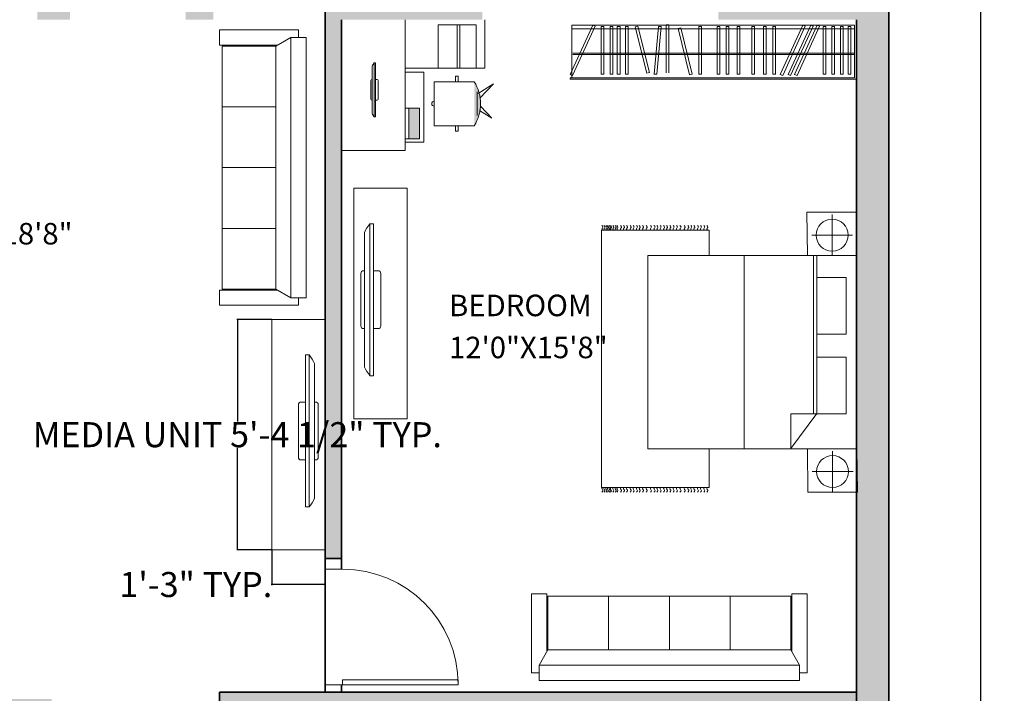
# Model space of a CAD drawing. Units: inches. Extents: x 1319 to 2030, y 219 to 1069.
# Tile 27 of 28: x 1727 to 2002, y 663 to 852. Entities that reach past the tile are written whole.
import ezdxf

# ---------------------------------------------------------------- set-up
doc = ezdxf.new("R2010")
doc.units = ezdxf.units.IN
doc.header["$MEASUREMENT"] = 0
doc.layers.get('0').update_dxf_attribs({"color": 12})
for name, color, linetype, lineweight in [('A-ANNO-DIMS', 2, 'Continuous', 18), ('A-AREA-IDEN', 250, 'Continuous', 18), ('A-WALL-PATT', 252, 'Continuous', 13), ('C-PROP', 7, 'Continuous', 35), ('closet', 252, 'Continuous', 18), ('doors', 252, 'Continuous', 18), ('furniture', 250, 'Continuous', 18), ('walls', 250, 'Continuous', 35)]:
    doc.layers.add(name, color=color, linetype=linetype, lineweight=lineweight)
doc.styles.get("Standard").update_dxf_attribs({"font": 'arial.ttf'})
doc.dimstyles.get("Standard").update_dxf_attribs({"dimtxt": 7, "dimasz": 0.18, "dimexe": 0.18, "dimexo": 0.0625, "dimgap": 0.09, "dimtad": 0, "dimtih": 1, "dimtoh": 1, "dimzin": 0, "dimdsep": 46, "dimlunit": 3, "dimtxsty": 'Standard', "dimcen": 0.09, "dimadec": 0, "dimazin": 0, "dimtfac": 1, "dimtofl": 0, "dimtmove": 0, "dimatfit": 3, "dimfxl": 1, "dimtolj": 1, "dimtzin": 0, "dimarcsym": 0})

# ---------------------------------------------------------------- blocks, each defined once
blk = doc.blocks.new('*U2')
for p, q in [((0, 0), (0, -6)), ((40, 0), (40, -6))]:
    blk.add_line(p, q)
blk.add_lwpolyline([(0, 0), (0, 40), (1.75, 40), (1.75, 0)], close=True)
blk.add_arc((0, 0), 40, 0, 90)
blk = doc.blocks.new('CARPET')
at = {"layer": 'furniture'}
for p, q in [((-51.53, -98.11), (-51.53, -55.12)), ((-51.53, -55.12), (-41.27, -55.12)), ((36, -55.12), (51.55, -55.12)), ((51.55, -55.12), (51.55, -98.11)), ((51.55, -98.11), (-51.53, -98.11))]:
    blk.add_line(p, q, dxfattribs=at)
for points, knots in [([(-53.37, -55.99), (-53.22, -55.8), (-52.9, -55.41), (-52.34, -55.8), (-51.89, -56.08), (-51.65, -55.91), (-51.53, -55.83)], [0, 0, 0, 0, 0.653278, 1.290138, 1.740457, 2.114451, 2.114451, 2.114451, 2.114451]), ([(-53.37, -57.26), (-53.22, -57.07), (-52.9, -56.67), (-52.34, -57.07), (-51.89, -57.35), (-51.65, -57.17), (-51.53, -57.1)], [0, 0, 0, 0, 0.653278, 1.290138, 1.740457, 2.114451, 2.114451, 2.114451, 2.114451]), ([(-53.37, -58.59), (-53.22, -58.4), (-52.9, -58.01), (-52.34, -58.4), (-51.89, -58.68), (-51.65, -58.5), (-51.53, -58.43)], [0, 0, 0, 0, 0.653278, 1.290138, 1.740457, 2.114451, 2.114451, 2.114451, 2.114451]), ([(53.37, -55.99), (53.22, -55.8), (52.9, -55.41), (52.34, -55.8), (51.89, -56.08), (51.65, -55.91), (51.53, -55.83)], [0, 0, 0, 0, 0.653278, 1.290138, 1.740457, 2.114451, 2.114451, 2.114451, 2.114451]), ([(53.37, -57.26), (53.22, -57.07), (52.9, -56.67), (52.34, -57.07), (51.89, -57.35), (51.65, -57.17), (51.53, -57.1)], [0, 0, 0, 0, 0.653278, 1.290138, 1.740457, 2.114451, 2.114451, 2.114451, 2.114451]), ([(53.37, -58.59), (53.22, -58.4), (52.9, -58.01), (52.34, -58.4), (51.89, -58.68), (51.65, -58.5), (51.53, -58.43)], [0, 0, 0, 0, 0.653278, 1.290138, 1.740457, 2.114451, 2.114451, 2.114451, 2.114451]), ([(-53.37, -59.78), (-53.22, -59.58), (-52.9, -59.19), (-52.34, -59.58), (-51.89, -59.86), (-51.65, -59.69), (-51.53, -59.61)], [0, 0, 0, 0, 0.653278, 1.290138, 1.740457, 2.114451, 2.114451, 2.114451, 2.114451]), ([(-53.37, -61.22), (-53.22, -61.02), (-52.9, -60.63), (-52.34, -61.02), (-51.89, -61.3), (-51.65, -61.13), (-51.53, -61.05)], [0, 0, 0, 0, 0.653278, 1.290138, 1.740457, 2.114451, 2.114451, 2.114451, 2.114451]), ([(-53.37, -62.44), (-53.22, -62.25), (-52.9, -61.86), (-52.34, -62.25), (-51.89, -62.53), (-51.65, -62.36), (-51.53, -62.28)], [0, 0, 0, 0, 0.653278, 1.290138, 1.740457, 2.114451, 2.114451, 2.114451, 2.114451]), ([(53.37, -59.78), (53.22, -59.58), (52.9, -59.19), (52.34, -59.58), (51.89, -59.86), (51.65, -59.69), (51.53, -59.61)], [0, 0, 0, 0, 0.653278, 1.290138, 1.740457, 2.114451, 2.114451, 2.114451, 2.114451]), ([(53.37, -61.22), (53.22, -61.02), (52.9, -60.63), (52.34, -61.02), (51.89, -61.3), (51.65, -61.13), (51.53, -61.05)], [0, 0, 0, 0, 0.653278, 1.290138, 1.740457, 2.114451, 2.114451, 2.114451, 2.114451]), ([(53.37, -62.44), (53.22, -62.25), (52.9, -61.86), (52.34, -62.25), (51.89, -62.53), (51.65, -62.36), (51.53, -62.28)], [0, 0, 0, 0, 0.653278, 1.290138, 1.740457, 2.114451, 2.114451, 2.114451, 2.114451]), ([(-53.37, -63.63), (-53.22, -63.43), (-52.9, -63.04), (-52.34, -63.43), (-51.89, -63.72), (-51.65, -63.54), (-51.53, -63.46)], [0, 0, 0, 0, 0.653278, 1.290138, 1.740457, 2.114451, 2.114451, 2.114451, 2.114451]), ([(-53.37, -65.07), (-53.22, -64.87), (-52.9, -64.48), (-52.34, -64.87), (-51.89, -65.15), (-51.65, -64.98), (-51.53, -64.9)], [0, 0, 0, 0, 0.653278, 1.290138, 1.740457, 2.114451, 2.114451, 2.114451, 2.114451]), ([(-53.37, -66.76), (-53.22, -66.56), (-52.9, -66.17), (-52.34, -66.56), (-51.89, -66.84), (-51.65, -66.67), (-51.53, -66.59)], [0, 0, 0, 0, 0.653278, 1.290138, 1.740457, 2.114451, 2.114451, 2.114451, 2.114451]), ([(53.37, -63.63), (53.22, -63.43), (52.9, -63.04), (52.34, -63.43), (51.89, -63.72), (51.65, -63.54), (51.53, -63.46)], [0, 0, 0, 0, 0.653278, 1.290138, 1.740457, 2.114451, 2.114451, 2.114451, 2.114451]), ([(53.37, -65.07), (53.22, -64.87), (52.9, -64.48), (52.34, -64.87), (51.89, -65.15), (51.65, -64.98), (51.53, -64.9)], [0, 0, 0, 0, 0.653278, 1.290138, 1.740457, 2.114451, 2.114451, 2.114451, 2.114451]), ([(53.37, -66.76), (53.22, -66.56), (52.9, -66.17), (52.34, -66.56), (51.89, -66.84), (51.65, -66.67), (51.53, -66.59)], [0, 0, 0, 0, 0.653278, 1.290138, 1.740457, 2.114451, 2.114451, 2.114451, 2.114451]), ([(-53.37, -68.2), (-53.22, -68), (-52.9, -67.61), (-52.34, -68), (-51.89, -68.28), (-51.65, -68.11), (-51.53, -68.03)], [0, 0, 0, 0, 0.653278, 1.290138, 1.740457, 2.114451, 2.114451, 2.114451, 2.114451]), ([(-53.37, -69.53), (-53.22, -69.33), (-52.9, -68.94), (-52.34, -69.33), (-51.89, -69.61), (-51.65, -69.44), (-51.53, -69.36)], [0, 0, 0, 0, 0.653278, 1.290138, 1.740457, 2.114451, 2.114451, 2.114451, 2.114451]), ([(-53.37, -70.79), (-53.22, -70.6), (-52.9, -70.21), (-52.34, -70.6), (-51.89, -70.88), (-51.65, -70.7), (-51.53, -70.63)], [0, 0, 0, 0, 0.653278, 1.290138, 1.740457, 2.114451, 2.114451, 2.114451, 2.114451]), ([(53.37, -68.2), (53.22, -68), (52.9, -67.61), (52.34, -68), (51.89, -68.28), (51.65, -68.11), (51.53, -68.03)], [0, 0, 0, 0, 0.653278, 1.290138, 1.740457, 2.114451, 2.114451, 2.114451, 2.114451]), ([(53.37, -69.53), (53.22, -69.33), (52.9, -68.94), (52.34, -69.33), (51.89, -69.61), (51.65, -69.44), (51.53, -69.36)], [0, 0, 0, 0, 0.653278, 1.290138, 1.740457, 2.114451, 2.114451, 2.114451, 2.114451]), ([(53.37, -70.79), (53.22, -70.6), (52.9, -70.21), (52.34, -70.6), (51.89, -70.88), (51.65, -70.7), (51.53, -70.63)], [0, 0, 0, 0, 0.653278, 1.290138, 1.740457, 2.114451, 2.114451, 2.114451, 2.114451]), ([(-53.37, -72.12), (-53.22, -71.93), (-52.9, -71.54), (-52.34, -71.93), (-51.89, -72.21), (-51.65, -72.04), (-51.53, -71.96)], [0, 0, 0, 0, 0.653278, 1.290138, 1.740457, 2.114451, 2.114451, 2.114451, 2.114451]), ([(-53.37, -73.31), (-53.22, -73.11), (-52.9, -72.72), (-52.34, -73.11), (-51.89, -73.4), (-51.65, -73.22), (-51.53, -73.14)], [0, 0, 0, 0, 0.653278, 1.290138, 1.740457, 2.114451, 2.114451, 2.114451, 2.114451]), ([(-53.37, -74.75), (-53.22, -74.55), (-52.9, -74.16), (-52.34, -74.55), (-51.89, -74.83), (-51.65, -74.66), (-51.53, -74.58)], [0, 0, 0, 0, 0.653278, 1.290138, 1.740457, 2.114451, 2.114451, 2.114451, 2.114451]), ([(53.37, -72.12), (53.22, -71.93), (52.9, -71.54), (52.34, -71.93), (51.89, -72.21), (51.65, -72.04), (51.53, -71.96)], [0, 0, 0, 0, 0.653278, 1.290138, 1.740457, 2.114451, 2.114451, 2.114451, 2.114451]), ([(53.37, -73.31), (53.22, -73.11), (52.9, -72.72), (52.34, -73.11), (51.89, -73.4), (51.65, -73.22), (51.53, -73.14)], [0, 0, 0, 0, 0.653278, 1.290138, 1.740457, 2.114451, 2.114451, 2.114451, 2.114451]), ([(53.37, -74.75), (53.22, -74.55), (52.9, -74.16), (52.34, -74.55), (51.89, -74.83), (51.65, -74.66), (51.53, -74.58)], [0, 0, 0, 0, 0.653278, 1.290138, 1.740457, 2.114451, 2.114451, 2.114451, 2.114451]), ([(-53.37, -75.98), (-53.22, -75.78), (-52.9, -75.39), (-52.34, -75.78), (-51.89, -76.06), (-51.65, -75.89), (-51.53, -75.81)], [0, 0, 0, 0, 0.653278, 1.290138, 1.740457, 2.114451, 2.114451, 2.114451, 2.114451]), ([(-53.37, -77.16), (-53.22, -76.96), (-52.9, -76.57), (-52.34, -76.96), (-51.89, -77.25), (-51.65, -77.07), (-51.53, -76.99)], [0, 0, 0, 0, 0.653278, 1.290138, 1.740457, 2.114451, 2.114451, 2.114451, 2.114451]), ([(-53.37, -78.6), (-53.22, -78.4), (-52.9, -78.01), (-52.34, -78.4), (-51.89, -78.68), (-51.65, -78.51), (-51.53, -78.43)], [0, 0, 0, 0, 0.653278, 1.290138, 1.740457, 2.114451, 2.114451, 2.114451, 2.114451]), ([(53.37, -75.98), (53.22, -75.78), (52.9, -75.39), (52.34, -75.78), (51.89, -76.06), (51.65, -75.89), (51.53, -75.81)], [0, 0, 0, 0, 0.653278, 1.290138, 1.740457, 2.114451, 2.114451, 2.114451, 2.114451]), ([(53.37, -77.16), (53.22, -76.96), (52.9, -76.57), (52.34, -76.96), (51.89, -77.25), (51.65, -77.07), (51.53, -76.99)], [0, 0, 0, 0, 0.653278, 1.290138, 1.740457, 2.114451, 2.114451, 2.114451, 2.114451]), ([(53.37, -78.6), (53.22, -78.4), (52.9, -78.01), (52.34, -78.4), (51.89, -78.68), (51.65, -78.51), (51.53, -78.43)], [0, 0, 0, 0, 0.653278, 1.290138, 1.740457, 2.114451, 2.114451, 2.114451, 2.114451]), ([(-53.37, -80.29), (-53.22, -80.09), (-52.9, -79.7), (-52.34, -80.09), (-51.89, -80.37), (-51.65, -80.2), (-51.53, -80.12)], [0, 0, 0, 0, 0.653278, 1.290138, 1.740457, 2.114451, 2.114451, 2.114451, 2.114451]), ([(-53.37, -81.73), (-53.22, -81.53), (-52.9, -81.14), (-52.34, -81.53), (-51.89, -81.81), (-51.65, -81.64), (-51.53, -81.56)], [0, 0, 0, 0, 0.653278, 1.290138, 1.740457, 2.114451, 2.114451, 2.114451, 2.114451]), ([(-53.37, -83.06), (-53.22, -82.86), (-52.9, -82.47), (-52.34, -82.86), (-51.89, -83.14), (-51.65, -82.97), (-51.53, -82.89)], [0, 0, 0, 0, 0.653278, 1.290138, 1.740457, 2.114451, 2.114451, 2.114451, 2.114451]), ([(53.37, -80.29), (53.22, -80.09), (52.9, -79.7), (52.34, -80.09), (51.89, -80.37), (51.65, -80.2), (51.53, -80.12)], [0, 0, 0, 0, 0.653278, 1.290138, 1.740457, 2.114451, 2.114451, 2.114451, 2.114451]), ([(53.37, -81.73), (53.22, -81.53), (52.9, -81.14), (52.34, -81.53), (51.89, -81.81), (51.65, -81.64), (51.53, -81.56)], [0, 0, 0, 0, 0.653278, 1.290138, 1.740457, 2.114451, 2.114451, 2.114451, 2.114451]), ([(53.37, -83.06), (53.22, -82.86), (52.9, -82.47), (52.34, -82.86), (51.89, -83.14), (51.65, -82.97), (51.53, -82.89)], [0, 0, 0, 0, 0.653278, 1.290138, 1.740457, 2.114451, 2.114451, 2.114451, 2.114451]), ([(-53.37, -84.18), (-53.22, -83.99), (-52.9, -83.6), (-52.34, -83.99), (-51.89, -84.27), (-51.65, -84.09), (-51.53, -84.02)], [0, 0, 0, 0, 0.653278, 1.290138, 1.740457, 2.114451, 2.114451, 2.114451, 2.114451]), ([(-53.37, -85.51), (-53.22, -85.32), (-52.9, -84.93), (-52.34, -85.32), (-51.89, -85.6), (-51.65, -85.42), (-51.53, -85.35)], [0, 0, 0, 0, 0.653278, 1.290138, 1.740457, 2.114451, 2.114451, 2.114451, 2.114451]), ([(-53.37, -86.7), (-53.22, -86.5), (-52.9, -86.11), (-52.34, -86.5), (-51.89, -86.78), (-51.65, -86.61), (-51.53, -86.53)], [0, 0, 0, 0, 0.653278, 1.290138, 1.740457, 2.114451, 2.114451, 2.114451, 2.114451]), ([(53.37, -84.18), (53.22, -83.99), (52.9, -83.6), (52.34, -83.99), (51.89, -84.27), (51.65, -84.09), (51.53, -84.02)], [0, 0, 0, 0, 0.653278, 1.290138, 1.740457, 2.114451, 2.114451, 2.114451, 2.114451]), ([(53.37, -85.51), (53.22, -85.32), (52.9, -84.93), (52.34, -85.32), (51.89, -85.6), (51.65, -85.42), (51.53, -85.35)], [0, 0, 0, 0, 0.653278, 1.290138, 1.740457, 2.114451, 2.114451, 2.114451, 2.114451]), ([(53.37, -86.7), (53.22, -86.5), (52.9, -86.11), (52.34, -86.5), (51.89, -86.78), (51.65, -86.61), (51.53, -86.53)], [0, 0, 0, 0, 0.653278, 1.290138, 1.740457, 2.114451, 2.114451, 2.114451, 2.114451]), ([(-53.37, -88.14), (-53.22, -87.94), (-52.9, -87.55), (-52.34, -87.94), (-51.89, -88.22), (-51.65, -88.05), (-51.53, -87.97)], [0, 0, 0, 0, 0.653278, 1.290138, 1.740457, 2.114451, 2.114451, 2.114451, 2.114451]), ([(-53.37, -89.36), (-53.22, -89.17), (-52.9, -88.78), (-52.34, -89.17), (-51.89, -89.45), (-51.65, -89.28), (-51.53, -89.2)], [0, 0, 0, 0, 0.653278, 1.290138, 1.740457, 2.114451, 2.114451, 2.114451, 2.114451]), ([(-53.37, -90.55), (-53.22, -90.35), (-52.9, -89.96), (-52.34, -90.35), (-51.89, -90.64), (-51.65, -90.46), (-51.53, -90.38)], [0, 0, 0, 0, 0.653278, 1.290138, 1.740457, 2.114451, 2.114451, 2.114451, 2.114451]), ([(53.37, -88.14), (53.22, -87.94), (52.9, -87.55), (52.34, -87.94), (51.89, -88.22), (51.65, -88.05), (51.53, -87.97)], [0, 0, 0, 0, 0.653278, 1.290138, 1.740457, 2.114451, 2.114451, 2.114451, 2.114451]), ([(53.37, -89.36), (53.22, -89.17), (52.9, -88.78), (52.34, -89.17), (51.89, -89.45), (51.65, -89.28), (51.53, -89.2)], [0, 0, 0, 0, 0.653278, 1.290138, 1.740457, 2.114451, 2.114451, 2.114451, 2.114451]), ([(53.37, -90.55), (53.22, -90.35), (52.9, -89.96), (52.34, -90.35), (51.9, -90.63), (51.66, -90.47), (51.55, -90.4)], [0, 0, 0, 0, 0.653278, 1.290138, 1.740457, 2.0926, 2.0926, 2.0926, 2.0926]), ([(-53.37, -91.99), (-53.22, -91.79), (-52.9, -91.4), (-52.34, -91.79), (-51.89, -92.07), (-51.65, -91.9), (-51.53, -91.82)], [0, 0, 0, 0, 0.653278, 1.290138, 1.740457, 2.114451, 2.114451, 2.114451, 2.114451]), ([(-53.37, -92.69), (-53.22, -92.48), (-52.9, -92.08), (-52.35, -92.49), (-51.89, -92.77), (-51.65, -92.6), (-51.53, -92.52)], [0, 0, 0, 0, 0.663904, 1.307406, 1.757725, 2.131719, 2.131719, 2.131719, 2.131719]), ([(-53.37, -93.61), (-53.22, -93.42), (-52.9, -93.03), (-52.34, -93.42), (-51.89, -93.7), (-51.65, -93.52), (-51.53, -93.45)], [0, 0, 0, 0, 0.653278, 1.290138, 1.740457, 2.114451, 2.114451, 2.114451, 2.114451]), ([(-53.37, -94.55), (-53.22, -94.35), (-52.9, -93.96), (-52.34, -94.35), (-51.89, -94.63), (-51.65, -94.46), (-51.53, -94.38)], [0, 0, 0, 0, 0.653278, 1.290138, 1.740457, 2.114451, 2.114451, 2.114451, 2.114451]), ([(53.37, -91.99), (53.22, -91.79), (52.9, -91.4), (52.34, -91.79), (51.9, -92.07), (51.66, -91.91), (51.55, -91.83)], [0, 0, 0, 0, 0.653278, 1.290138, 1.740457, 2.0926, 2.0926, 2.0926, 2.0926]), ([(53.37, -92.69), (53.22, -92.49), (52.9, -92.09), (52.34, -92.49), (51.9, -92.77), (51.66, -92.61), (51.55, -92.53)], [0, 0, 0, 0, 0.656792, 1.295826, 1.746145, 2.098292, 2.098292, 2.098292, 2.098292]), ([(53.37, -93.66), (53.22, -93.46), (52.9, -93.07), (52.34, -93.46), (51.9, -93.74), (51.66, -93.58), (51.55, -93.5)], [0, 0, 0, 0, 0.653278, 1.290138, 1.740457, 2.0926, 2.0926, 2.0926, 2.0926]), ([(53.37, -94.59), (53.22, -94.4), (52.9, -94.01), (52.34, -94.4), (51.9, -94.68), (51.66, -94.51), (51.55, -94.44)], [0, 0, 0, 0, 0.653278, 1.290138, 1.740457, 2.0926, 2.0926, 2.0926, 2.0926]), ([(-53.37, -95.05), (-53.22, -94.85), (-52.9, -94.46), (-52.34, -94.85), (-51.89, -95.14), (-51.65, -94.96), (-51.53, -94.88)], [0, 0, 0, 0, 0.653278, 1.290138, 1.740457, 2.114451, 2.114451, 2.114451, 2.114451]), ([(-53.37, -95.73), (-53.22, -95.54), (-52.9, -95.15), (-52.34, -95.54), (-51.89, -95.82), (-51.65, -95.65), (-51.53, -95.57)], [0, 0, 0, 0, 0.653278, 1.290138, 1.740457, 2.114451, 2.114451, 2.114451, 2.114451]), ([(-53.37, -96.38), (-53.22, -96.18), (-52.9, -95.79), (-52.34, -96.18), (-51.89, -96.47), (-51.65, -96.29), (-51.53, -96.21)], [0, 0, 0, 0, 0.653278, 1.290138, 1.740457, 2.114451, 2.114451, 2.114451, 2.114451]), ([(-53.37, -97.17), (-53.22, -96.98), (-52.9, -96.59), (-52.34, -96.98), (-51.89, -97.26), (-51.65, -97.08), (-51.53, -97.01)], [0, 0, 0, 0, 0.653278, 1.290138, 1.740457, 2.114451, 2.114451, 2.114451, 2.114451]), ([(-53.37, -97.99), (-53.22, -97.79), (-52.9, -97.4), (-52.34, -97.79), (-51.89, -98.08), (-51.65, -97.9), (-51.53, -97.82)], [0, 0, 0, 0, 0.653278, 1.290138, 1.740457, 2.114451, 2.114451, 2.114451, 2.114451]), ([(53.37, -95.78), (53.22, -95.58), (52.9, -95.19), (52.34, -95.58), (51.89, -95.86), (51.65, -95.69), (51.53, -95.61)], [0, 0, 0, 0, 0.653278, 1.290138, 1.740457, 2.114451, 2.114451, 2.114451, 2.114451]), ([(53.37, -96.43), (53.22, -96.23), (52.9, -95.84), (52.34, -96.23), (51.89, -96.51), (51.65, -96.34), (51.53, -96.26)], [0, 0, 0, 0, 0.653278, 1.290138, 1.740457, 2.114451, 2.114451, 2.114451, 2.114451]), ([(53.37, -97.22), (53.22, -97.02), (52.9, -96.63), (52.34, -97.02), (51.89, -97.3), (51.65, -97.13), (51.53, -97.05)], [0, 0, 0, 0, 0.653278, 1.290138, 1.740457, 2.114451, 2.114451, 2.114451, 2.114451]), ([(53.37, -97.99), (53.22, -97.79), (52.9, -97.4), (52.34, -97.79), (51.89, -98.08), (51.65, -97.9), (51.53, -97.82)], [0, 0, 0, 0, 0.653278, 1.290138, 1.740457, 2.114451, 2.114451, 2.114451, 2.114451]), ([(53.37, -95.1), (53.22, -94.9), (52.9, -94.51), (52.34, -94.9), (51.9, -95.18), (51.66, -95.02), (51.55, -94.94)], [0, 0, 0, 0, 0.653278, 1.290138, 1.740457, 2.0926, 2.0926, 2.0926, 2.0926])]:
    blk.add_open_spline(points, degree=3, knots=knots, dxfattribs=at)
blk = doc.blocks.new('A$C58D270C6')
at = {"layer": 'furniture'}
for p, q in [((9.09, 124.13), (9.09, 108.87)), ((1.46, 116.5), (16.73, 116.5)), ((14.97, 94.84), (24.62, 107.92)), ((24.62, 94.93), (24.62, 107.92)), ((42.08, 108), (42.08, 36)), ((14.97, 94.93), (24.62, 94.93)), ((14.97, 94.84), (14.97, 36)), ((16.22, 94.93), (16.22, 36)), ((9.25, 36), (9.25, 20.74)), ((1.62, 28.37), (16.88, 28.37))]:
    blk.add_line(p, q, dxfattribs=at)
for points in [[(18.5, 108), (18.34, 124.13), (-0.16, 124.13), (0, 108)], [(0, 108), (77.91, 108), (77.91, 36), (0, 36)], [(4.09, 94.93), (14.97, 94.93), (14.97, 73.83), (4.09, 73.83)], [(4.09, 65.23), (14.97, 65.23), (14.97, 44.13), (4.09, 44.13)], [(18.65, 19.87), (18.5, 36), (0, 36), (0.16, 19.87)]]:
    blk.add_lwpolyline(points, close=True, dxfattribs=at)
for centre in [(9.09, 116.5), (9.25, 28.37)]:
    blk.add_circle(centre, 5.95, dxfattribs=at)
at = {"layer": 'furniture', "xscale": 0.9312884925094044, "yscale": 0.9312884925094044, "zscale": 0.9312884925094044, "rotation": 90}
blk.add_blockref('CARPET', (3.79, 74.47), dxfattribs=at)
blk = doc.blocks.new('FABRIC SOFA 4S')
at = {"layer": 'furniture'}
for p, q in [((0, -51), (0, 51)), ((6, 51), (0, 51)), ((3, 54), (34, 54)), ((3, 51), (3, 54)), ((6, -51), (6, 51)), ((12, 47.63), (6, 51)), ((34, 48), (34, 54)), ((11.14, 48), (34, 48)), ((33, 23.81), (12, 23.81)), ((33, 0), (12, 0)), ((33, -23.81), (12, -23.81)), ((6, -51), (12, -47.63)), ((11.54, -48), (34, -48)), ((34, -48), (34, -54)), ((6, -51), (0, -51)), ((3, -54), (3, -51)), ((3, -54), (34, -54))]:
    blk.add_line(p, q, dxfattribs=at)
blk.add_lwpolyline([(12, -47.63), (12, 47.63), (33, 47.63), (33, -47.63)], close=True, dxfattribs=at)
blk = doc.blocks.new('*D29')
at = {"layer": 'A-ANNO-DIMS', "color": 0, "lineweight": -2, "transparency": 16777216}
for p, q in [((1995.58, 955.23), (1995.33, 955.23)), ((1995.51, 955.05), (1995.51, 628.88)), ((1995.51, 295.41), (1995.51, 621.58)), ((1995.58, 295.23), (1995.33, 295.23))]:
    blk.add_line(p, q, dxfattribs=at)
at = {"layer": 'A-ANNO-DIMS', "color": 0, "transparency": 16777216}
for points in [[(1995.48, 955.05), (1995.54, 955.05), (1995.51, 955.23)], [(1995.48, 295.41), (1995.54, 295.41), (1995.51, 295.23)]]:
    blk.add_solid(points, dxfattribs=at)
at = {"layer": 'Defpoints', "color": 0, "transparency": 16777216}
for p in [(1995.64, 955.23), (1995.51, 295.23), (1995.64, 295.23)]:
    blk.add_point(p, dxfattribs=at)
at = {"layer": 'A-ANNO-DIMS', "color": 0, "transparency": 16777216, "insert": (1995.51, 625.23), "char_height": 7, "attachment_point": 5}
blk.add_mtext("\\A1;55'", dxfattribs=at)
blk = doc.blocks.new('PLASMA-LARGE')
at = {"layer": 'furniture'}
for p, q in [((-7.26, 0), (7.26, 0)), ((-21, -2.5), (21, -2.5)), ((-21, -2.5), (-21, -3.5)), ((-18.61, -1), (18.61, -1)), ((-8, -1), (-8, -0.74)), ((8, -1), (8, -0.74)), ((21, -2.5), (21, -3.5)), ((-21, -3.5), (21, -3.5)), ((-8, -3.5), (-8, -4.76)), ((8, -3.5), (8, -4.76)), ((-7.26, -5.5), (7.26, -5.5))]:
    blk.add_line(p, q, dxfattribs=at)
for centre, radius, start, end in [((-7.26, -0.74), 0.744, 90, 180), ((7.26, -0.74), 0.744, 0, 90), ((-13.97, -11.05), 11.07, 114.7602, 129.4175), ((13.97, -11.05), 11.07, 50.5825, 65.2398), ((-7.26, -4.76), 0.744, 180, 270), ((7.26, -4.76), 0.744, 270, 0)]:
    blk.add_arc(centre, radius, start, end, dxfattribs=at)
blk = doc.blocks.new('STUDY-STATION')
h = blk.add_hatch(color=256)
h.dxf.hatch_style = 1
h.paths.add_polyline_path([(29.65, 37, 0.288578), (17.34, 37)])
h = blk.add_hatch(color=256)
h.dxf.hatch_style = 1
h.paths.add_polyline_path([(33.33, 21.74), (24.73, 21.74), (24.73, 18.77), (33.33, 18.77)])
for p, q in [((20.6, 38.07), (17.92, 42.38)), ((17.92, 42.38), (21.92, 38.58)), ((27.56, 41.97), (24.23, 38.82)), ((25.39, 38.48), (27.56, 41.97)), ((13.58, 39.93), (0, 39.93)), ((13.58, 17.73), (13.58, 39.93)), ((13.58, 37.53), (1.44, 37.53)), ((1.44, 37.53), (1.44, 26.9)), ((17.34, 37), (17.34, 25.83)), ((26.82, 37.82), (20.17, 37.82)), ((29.65, 25.83), (29.65, 37)), ((13.58, 32.99), (1.44, 32.99)), ((1.44, 32.99), (1.44, 32.21)), ((1.44, 32.21), (13.58, 32.21)), ((13.58, 26.9), (13.58, 32.99)), ((17.34, 32.49), (15.81, 32.49)), ((15.81, 32.49), (15.81, 31.73)), ((15.81, 31.73), (17.34, 31.73)), ((17.34, 32.49), (17.34, 32.49)), ((29.65, 32.49), (31.18, 32.49)), ((31.18, 31.73), (29.65, 31.73)), ((31.18, 32.49), (31.18, 31.73)), ((1.44, 26.9), (13.58, 26.9)), ((17.34, 25.83), (29.65, 25.83)), ((14.64, 17.73), (14.64, 22.88)), ((14.64, 22.88), (34.27, 22.88)), ((34.27, 22.88), (34.27, 17.73)), ((24.73, 17.73), (24.73, 21.74)), ((24.73, 21.74), (33.33, 21.74)), ((33.33, 21.74), (33.33, 17.73)), ((0, 17.73), (36.53, 17.73)), ((24.73, 18.77), (33.33, 18.77)), ((36.53, 17.73), (36.53, 0))]:
    blk.add_line(p, q)
for centre, radius, start, end in [((23.49, 27.23), 11.55, 57.806, 122.194), ((23.49, 25.83), 0.688, 180, 0)]:
    blk.add_arc(centre, radius, start, end)
at = {"xscale": -0.3577737849257557, "yscale": 0.3577737849257557, "zscale": 0.3577737849257557, "rotation": 180}
blk.add_blockref('PLASMA-LARGE', (19.61, 8.15), dxfattribs=at)
blk = doc.blocks.new('MEDIA-CONSOLE')
for p, q in [((64.44, 14.9), (0, 14.9)), ((0, 14.9), (0, 0)), ((64.44, 0), (64.44, 14.9)), ((0, 0), (64.44, 0))]:
    blk.add_line(p, q)
at = {"xscale": -1.011294184530666, "yscale": 1.011294184530666, "zscale": 1.011294184530666, "rotation": 180}
blk.add_blockref('PLASMA-LARGE', (33.26, 1.95), dxfattribs=at)
blk = doc.blocks.new('closet')
at = {"layer": 'closet'}
for p, q in [((-0.71, -5.58), (5.59, 8.19)), ((-0.23, 7.39), (-0.23, -6.57)), ((6.27, 7.88), (-0.04, -5.89)), ((5.59, 8.19), (6.27, 7.88)), ((7.92, 7.84), (8.68, 7.84)), ((7.92, 7.84), (7.92, -5.51)), ((8.68, 7.84), (8.68, -5.51)), ((10.44, 7.84), (11.2, 7.84)), ((10.44, 7.84), (10.44, -5.51)), ((11.2, 7.84), (11.2, -5.51)), ((12.45, 7.84), (13.21, 7.84)), ((12.45, 7.84), (12.45, -5.51)), ((13.21, 7.84), (13.21, -5.51)), ((14.71, 7.84), (15.47, 7.84)), ((14.71, 7.84), (14.71, -5.51)), ((15.47, 7.84), (15.47, -5.51)), ((17.44, 7.75), (18.17, 7.93)), ((17.44, 7.75), (20.73, -5.2)), ((18.17, 7.93), (21.46, -5.01)), ((23.92, 7.84), (22.75, -5.46)), ((24.67, 7.78), (23.51, -5.53)), ((23.92, 7.84), (24.67, 7.78)), ((26.09, 8.25), (26.09, -5.1)), ((26.84, 8.25), (26.84, -5.1)), ((29.49, 7.29), (32.64, -5.69)), ((30.22, 7.46), (33.37, -5.51)), ((35.23, 7.84), (35.23, -5.51)), ((35.99, 7.84), (35.99, -5.51)), ((40.33, 7.84), (40.33, -5.51)), ((41.08, 7.84), (41.08, -5.51)), ((42.85, 7.84), (42.85, -5.51)), ((43.61, 7.84), (43.61, -5.51)), ((45.9, 7.84), (45.9, -5.51)), ((46.65, 7.84), (46.65, -5.51)), ((50.07, 7.84), (50.07, -5.51)), ((50.82, 7.84), (50.82, -5.51)), ((53.32, 7.84), (53.32, -5.51)), ((54.08, 7.84), (54.08, -5.51)), ((55.9, 7.84), (55.9, -5.51)), ((56.65, 7.84), (56.65, -5.51)), ((57.99, -5.58), (64.3, 8.19)), ((64.97, 7.88), (58.67, -5.89)), ((60.19, -5.58), (66.49, 8.19)), ((67.17, 7.88), (60.87, -5.89)), ((62, -5.58), (68.3, 8.19)), ((68.98, 7.88), (62.67, -5.89)), ((69.96, 7.84), (69.96, -5.51)), ((70.72, 7.84), (70.72, -5.51)), ((72.43, 7.84), (72.43, -5.51)), ((73.19, 7.84), (73.19, -5.51)), ((74.82, 7.84), (74.82, -5.51)), ((75.57, 7.84), (75.57, -5.51)), ((76.94, 7.84), (76.94, -5.51)), ((77.69, 7.84), (77.69, -5.51)), ((56.23, 0.33), (0, 0.33)), ((56.2, 0), (0, 0)), ((56.2, 0), (78.76, 0)), ((56.23, 0.33), (78.76, 0.33)), ((21.46, -5.01), (20.73, -5.2)), ((23.51, -5.53), (22.75, -5.46)), ((-0.04, -5.89), (-0.71, -5.58)), ((33.37, -5.51), (32.64, -5.69)), ((35.99, -5.51), (35.23, -5.51)), ((41.08, -5.51), (40.33, -5.51)), ((43.61, -5.51), (42.85, -5.51)), ((46.65, -5.51), (45.9, -5.51)), ((50.82, -5.51), (50.07, -5.51)), ((54.08, -5.51), (53.32, -5.51)), ((56.65, -5.51), (55.9, -5.51)), ((58.67, -5.89), (57.99, -5.58)), ((60.87, -5.89), (60.19, -5.58)), ((62.67, -5.89), (62, -5.58)), ((70.72, -5.51), (69.96, -5.51)), ((73.19, -5.51), (72.43, -5.51)), ((75.57, -5.51), (74.82, -5.51)), ((77.69, -5.51), (76.94, -5.51))]:
    blk.add_line(p, q, dxfattribs=at)
blk = doc.blocks.new('rotated closet')
at = {"layer": 'closet'}
for p, q in [((26.32, 0.86), (27.07, 0.86)), ((29.72, -0.11), (30.45, 0.07)), ((35.46, 0.45), (36.22, 0.45)), ((40.56, 0.45), (41.31, 0.45)), ((43.08, 0.45), (43.84, 0.45)), ((46.13, 0.45), (46.88, 0.45)), ((50.3, 0.45), (51.05, 0.45)), ((53.56, 0.45), (54.31, 0.45)), ((56.13, 0.45), (56.88, 0.45)), ((64.53, 0.8), (65.2, 0.49)), ((66.72, 0.8), (67.4, 0.49)), ((68.53, 0.8), (69.21, 0.49)), ((70.19, 0.45), (70.95, 0.45)), ((72.66, 0.45), (73.42, 0.45)), ((75.05, 0.45), (75.81, 0.45)), ((77.17, 0.45), (77.92, 0.45)), ((78.99, 0), (78.99, -13.96)), ((8.91, -12.91), (8.15, -12.91)), ((11.43, -12.91), (10.67, -12.91)), ((13.44, -12.91), (12.68, -12.91)), ((15.7, -12.91), (14.94, -12.91)), ((-0.46, -14.27), (79.54, -14.27)), ((0, -13.96), (78.99, -13.96))]:
    blk.add_line(p, q, dxfattribs=at)
blk.add_blockref('closet', (0.23, -7.39), dxfattribs=at)
blk = doc.blocks.new('WARDROBE-80')
for p, q in [((15.13, 0.02), (15.13, 80.02)), ((15.13, 0.02), (15.13, 80.02)), ((15.13, 0.02), (15.13, 80.02)), ((14.82, 79.47), (0.01, 79.47)), ((0.01, 0.48), (0.01, 79.47)), ((1.04, 79.35), (1.04, 0.36)), ((14.82, 0.48), (14.82, 79.47)), ((14.82, 0.48), (14.82, 77.83)), ((15.13, 77.37), (15.13, 79.47)), ((15.13, 77.37), (15.13, 79.47)), ((0.01, 0.48), (14.82, 0.48)), ((14.82, 0.02), (14.82, 0.48)), ((15.13, 0.02), (14.82, 0.02))]:
    blk.add_line(p, q)
at = {"rotation": 89.99999999920078}
blk.add_blockref('rotated closet', (0.86, 0.48), dxfattribs=at)
blk = doc.blocks.new('*D38')
at = {"layer": 'A-ANNO-DIMS', "color": 0, "lineweight": -2, "transparency": 16777216}
for p, q in [((1797.38, 767.84), (1787.6, 767.84)), ((1787.78, 767.66), (1787.78, 739.33)), ((1787.78, 703.58), (1787.78, 731.91)), ((1797.38, 703.4), (1787.6, 703.4))]:
    blk.add_line(p, q, dxfattribs=at)
at = {"layer": 'A-ANNO-DIMS', "color": 0, "transparency": 16777216}
for points in [[(1787.75, 767.66), (1787.81, 767.66), (1787.78, 767.84)], [(1787.75, 703.58), (1787.81, 703.58), (1787.78, 703.4)]]:
    blk.add_solid(points, dxfattribs=at)
at = {"layer": 'Defpoints', "color": 0, "transparency": 16777216}
for p in [(1787.78, 767.84), (1797.45, 767.84), (1797.45, 703.4)]:
    blk.add_point(p, dxfattribs=at)
at = {"layer": 'A-ANNO-DIMS', "color": 0, "transparency": 16777216, "insert": (1787.78, 735.62), "char_height": 7, "attachment_point": 5}
blk.add_mtext('\\A1;MEDIA UNIT 5\'-4 1/2" TYP.', dxfattribs=at)
blk = doc.blocks.new('*D39')
at = {"layer": 'A-ANNO-DIMS', "color": 0, "lineweight": -2, "transparency": 16777216}
for p, q in [((1797.45, 703.33), (1797.45, 693.55)), ((1812.34, 703.33), (1812.34, 693.55)), ((1797.45, 693.73), (1797.27, 693.73)), ((1812.16, 693.73), (1797.63, 693.73))]:
    blk.add_line(p, q, dxfattribs=at)
at = {"layer": 'A-ANNO-DIMS', "color": 0, "transparency": 16777216}
for points in [[(1797.63, 693.76), (1797.63, 693.7), (1797.45, 693.73)], [(1812.16, 693.76), (1812.16, 693.7), (1812.34, 693.73)]]:
    blk.add_solid(points, dxfattribs=at)
at = {"layer": 'Defpoints', "color": 0, "transparency": 16777216}
for p in [(1797.45, 703.4), (1812.34, 703.4), (1797.45, 693.73)]:
    blk.add_point(p, dxfattribs=at)
at = {"layer": 'A-ANNO-DIMS', "color": 0, "transparency": 16777216, "insert": (1776.17, 693.73), "char_height": 7, "attachment_point": 5}
blk.add_mtext('\\A1;1\'-3" TYP.', dxfattribs=at)

msp = doc.modelspace()

# ---------------------------------------------------------------- hatches: boundary and pattern name
at = {"layer": 'A-WALL-PATT'}
h = msp.add_hatch(color=256, dxfattribs=at)
h.dxf.hatch_style = 1
h.paths.add_polyline_path([(1378.843, 946.227), (1960.843, 946.227), (1960.843, 860.616), (1922.194, 860.616), (1922.194, 851.616), (1960.843, 851.616), (1960.843, 304.227), (1578.343, 304.227), (1578.343, 295.227), (1969.843, 295.227), (1969.843, 955.227), (1369.843, 955.227), (1369.843, 295.227), (1378.843, 295.227)])
h = msp.add_hatch(color=256, dxfattribs=at)
h.dxf.hatch_style = 1
h.paths.add_polyline_path([(1856.292, 860.616), (1812.343, 860.616), (1812.343, 851.616), (1812.343, 700.993), (1816.843, 700.993), (1816.843, 851.616), (1856.292, 851.616)])
h.paths.add_polyline_path([(1960.843, 663.616), (1812.343, 663.616), (1782.783, 663.616), (1782.783, 659.116), (1812.343, 659.116), (1960.843, 659.116)])
h.paths.add_polyline_path([(1857.424, 659.116), (1852.924, 659.116), (1852.924, 616.807), (1857.424, 616.807)])
h.paths.add_polyline_path([(1735.843, 661.727), (1731.843, 661.727), (1636.133, 661.727), (1636.133, 657.227), (1731.343, 657.227), (1731.343, 481.227), (1618.616, 481.227), (1618.616, 472.227), (1639.343, 472.227), (1639.343, 384.227), (1627.044, 384.227), (1627.044, 375.227), (1648.343, 375.227), (1648.343, 384.227), (1648.343, 472.227), (1750.706, 472.227), (1750.706, 481.227), (1735.843, 481.227), (1735.843, 657.727)])
h.paths.add_polyline_path([(1587.343, 481.227), (1578.343, 481.227), (1578.343, 375.227), (1597.622, 375.227), (1597.622, 384.227), (1587.343, 384.227)])
h.paths.add_polyline_path([(1769.593, 384.227), (1693.482, 384.227), (1693.482, 375.227), (1769.593, 375.227)])
h.paths.add_polyline_path([(1775.828, 481.227), (1765.831, 481.227), (1765.831, 472.227), (1775.828, 472.227)])
h.paths.add_polyline_path([(1824.625, 481.227), (1820.343, 481.227), (1820.343, 476.727), (1824.625, 476.727), (1824.625, 477.545)], flags=0)
h.paths.add_polyline_path([(1896.843, 481.227), (1852.26, 481.227), (1852.26, 476.727), (1892.343, 476.727), (1892.343, 384.227), (1881.742, 384.227), (1881.742, 375.227), (1913.435, 375.227), (1913.435, 384.227), (1896.843, 384.227)])
h.paths.add_polyline_path([(1960.843, 481.227), (1931.341, 481.227), (1931.341, 476.727), (1960.843, 476.727)])
h.paths.add_polyline_path([(1736.343, 918.227), (1731.843, 918.227), (1731.843, 890.227), (1582.843, 890.227), (1582.843, 781.727), (1582.843, 769.171), (1587.343, 769.171), (1587.343, 781.727), (1587.343, 885.727), (1731.843, 885.727), (1731.843, 851.616), (1736.343, 851.616), (1736.343, 890.227)])
h.paths.add_polyline_path([(1781.022, 860.616), (1773.021, 860.616, -0.0322281), (1773.289, 856.464), (1773.289, 851.616), (1781.022, 851.616)])
h.paths.add_polyline_path([(1587.343, 946.227), (1582.843, 946.227), (1582.843, 926.136), (1587.343, 926.136)])
h.paths.add_polyline_path([(1647.843, 946.227), (1643.343, 946.227), (1643.343, 926.136), (1647.843, 926.136)])
h.paths.add_polyline_path([(1543.343, 786.227), (1429.843, 786.227), (1429.843, 757.555), (1434.343, 757.555), (1438.843, 757.555), (1438.843, 781.727), (1543.343, 781.727)])
h.paths.add_polyline_path([(1543.343, 781.727), (1538.843, 781.727), (1538.843, 709.727), (1534.597, 709.727), (1534.597, 705.227), (1543.343, 705.227), (1543.343, 709.727)])
h.paths.add_polyline_path([(1499.955, 709.727), (1438.843, 709.727), (1438.843, 734.463), (1429.843, 734.463), (1429.843, 552.227), (1470.241, 552.227), (1470.241, 561.227), (1438.843, 561.227), (1438.843, 705.227), (1499.955, 705.227)])
h.paths.add_polyline_path([(1587.343, 709.727), (1582.843, 709.727), (1582.843, 561.227), (1543.433, 561.227), (1543.433, 552.227), (1587.343, 552.227)])
h.paths.add_polyline_path([(1546.835, 709.727), (1543.343, 709.727), (1543.343, 705.227), (1546.835, 705.227)])
h.paths.add_polyline_path([(1582.843, 709.727), (1579.15, 709.727), (1579.15, 705.227), (1582.843, 705.227)], flags=17)
h.paths.add_polyline_path([(1548.368, 786.227), (1543.343, 786.227), (1543.343, 781.727), (1548.368, 781.727)])
h.paths.add_polyline_path([(1582.843, 786.227), (1580.683, 786.227), (1580.683, 781.727), (1582.843, 781.727)])
h.paths.add_polyline_path([(1587.343, 892.402), (1582.843, 892.402), (1582.843, 890.227), (1587.343, 890.227)], flags=17)
h.paths.add_polyline_path([(1647.843, 892.402), (1643.343, 892.402), (1643.343, 890.227), (1647.843, 890.227)], flags=17)
h.paths.add_polyline_path([(1740.974, 856.464), (1740.974, 860.616), (1736.343, 860.616), (1736.343, 851.616), (1740.974, 851.616)])
h.paths.add_polyline_path([(1853.989, 384.227), (1820.343, 384.227), (1820.343, 402.924), (1815.843, 402.924), (1815.843, 375.227), (1853.989, 375.227)])
h.paths.add_polyline_path([(1892.343, 436.227), (1820.343, 436.227), (1820.343, 481.227), (1815.843, 481.227), (1815.843, 431.727), (1892.343, 431.727)])
h.paths.add_polyline_path([(1849.175, 481.227), (1824.625, 481.227), (1824.625, 477.545), (1825.699, 477.545), (1825.699, 453.018, 0.4014527), (1849.175, 477.545)], flags=0)
h.paths.add_polyline_path([(1960.843, 384.227), (1941.188, 384.227), (1941.188, 375.227), (1960.843, 375.227)])
h.paths.add_polyline_path([(1902.267, 481.227), (1896.843, 481.227), (1896.843, 476.727), (1902.267, 476.727), (1902.267, 477.44)], flags=0)

# ---------------------------------------------------------------- linework, layer by layer
at = {"layer": 'C-PROP'}
msp.add_line((1969.843, 955.227), (1969.843, 295.227), dxfattribs=at)
at = {"layer": 'walls'}
for p, q in [((1812.343, 860.616), (1812.343, 663.616)), ((1816.843, 851.616), (1816.843, 698.031)), ((1960.843, 851.616), (1960.843, 304.227)), ((1812.343, 700.993), (1816.843, 700.993)), ((1812.343, 663.616), (1782.783, 663.616)), ((1782.783, 663.616), (1782.783, 659.116)), ((1812.343, 663.616), (1960.843, 663.616)), ((1816.843, 665.716), (1816.843, 663.616))]:
    msp.add_line(p, q, dxfattribs=at)

# ---------------------------------------------------------------- block references
at = {"layer": 'closet', "rotation": 270.0000000040735}
msp.add_blockref('WARDROBE-80', (1880.819, 850.141), dxfattribs=at)
at = {"layer": 'doors', "xscale": -0.8078659498341503, "yscale": 0.8078659498341503, "zscale": 0.8078659498341503, "rotation": 270}
msp.add_blockref('*U2', (1817.19, 665.716), dxfattribs=at)
at = {"layer": 'furniture'}
for name, p, rotation in [('STUDY-STATION', (1816.976, 851.616), 269.9999999999988), ('MEDIA-CONSOLE', (1812.343, 703.396), 89.99999999999935)]:
    msp.add_blockref(name, p, dxfattribs=dict(at, rotation=rotation))
at = {"layer": 'furniture', "xscale": -0.7127038693416449, "yscale": 0.7127038693416449, "zscale": 0.7127038693416449}
msp.add_blockref('FABRIC SOFA 4S', (1807.042, 810.262), dxfattribs=at)
at = {"layer": 'furniture', "extrusion": (0, 0, -1), "zscale": -1, "rotation": 90.00000000000183}
msp.add_blockref('MEDIA-CONSOLE', (-1820.356, 740.088), dxfattribs=at)
at = {"layer": 'furniture'}
for name, p, xscale, yscale, zscale, rotation in [('A$C58D270C6', (1960.959, 812.68), 0.7500000390647866, 0.7500000390647866, 0.7500000390647866, 180), ('FABRIC SOFA 4S', (1908.517, 666.935), -0.7127038693416449, 0.7127038693416449, 0.7127038693416449, 270)]:
    msp.add_blockref(name, p, dxfattribs=dict(at, xscale=xscale, yscale=yscale, zscale=zscale, rotation=rotation))

# ---------------------------------------------------------------- texts
at = {"layer": 'A-AREA-IDEN'}
for s, height, p in [('19\'0"X18\'8"', 6.01124, (1697.378, 788.788)), ('BEDROOM', 6.0112, (1846.935, 768.738)), ('12\'0"X15\'8"', 6.01124, (1846.935, 756.989))]:
    msp.add_text(s, height=height, dxfattribs=at).set_placement(p)

# ---------------------------------------------------------------- dimensions: what is measured, and where the dimension line sits
at = {"layer": 'A-ANNO-DIMS'}
dim = msp.add_linear_dim(base=(1995.506, 295.227), p1=(1995.643, 955.227), p2=(1995.643, 295.227), angle=90, dimstyle='Standard', override={"dimclrd": 0, "dimclre": 0, "dimclrt": 0}, dxfattribs=at)
dim.commit()
dim.dimension.update_dxf_attribs({"geometry": '*D29', "text_midpoint": (1995.506, 625.227)})
for base, p1, p2, angle, text, picture, middle in [((1787.779, 767.839), (1797.446, 703.396), (1797.446, 767.839), 90, 'MEDIA UNIT <> TYP.', '*D38', (1787.779, 735.617)), ((1797.446, 693.729), (1812.343, 703.396), (1797.446, 703.396), 180, '<> TYP.', '*D39', (1776.171, 693.729))]:
    dim = msp.add_linear_dim(base=base, p1=p1, p2=p2, angle=angle, text=text, dimstyle='Standard', override={"dimdec": 1, "dimlfac": 1, "dimrnd": 0, "dimzin": 1, "dimdsep": 46, "dimlunit": 4, "dimfrac": 2}, dxfattribs=at)
    dim.commit()
    dim.dimension.update_dxf_attribs({"geometry": picture, "text_midpoint": middle})

doc.saveas('drawing.dxf')
